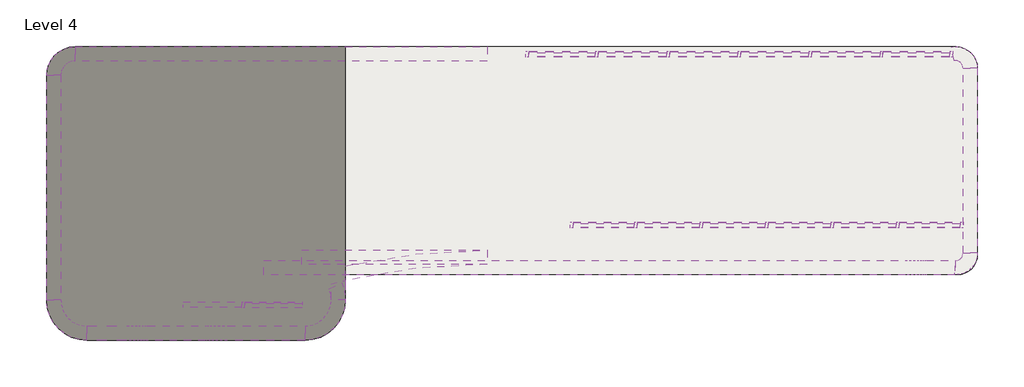
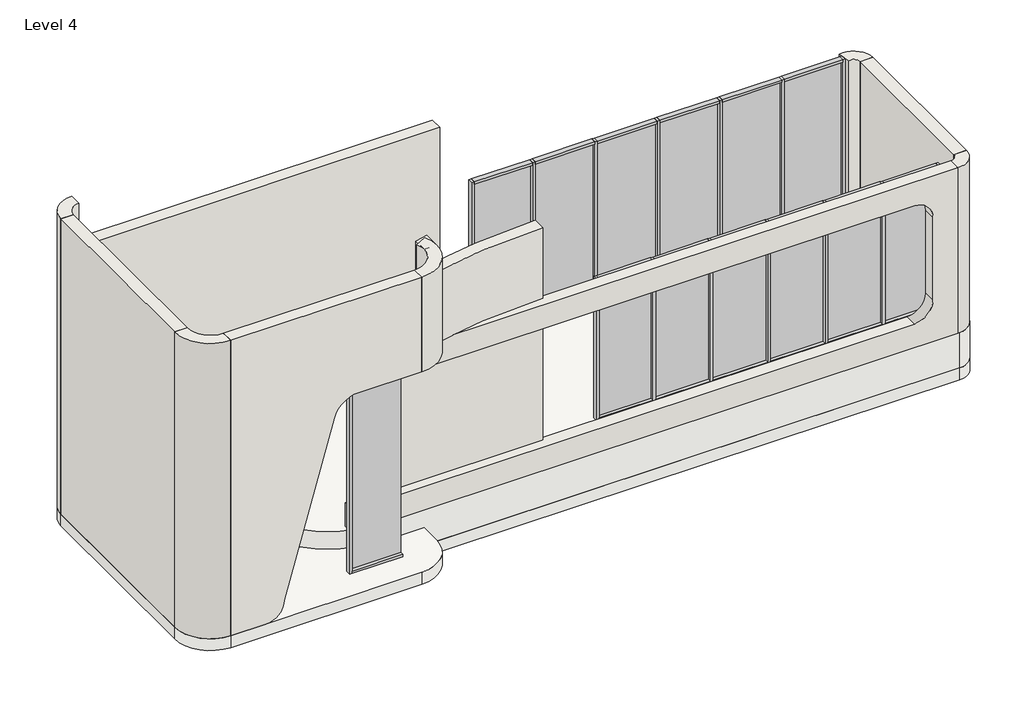
# One storey, incomplete: 41 members, 13 plates, 13 walls, 3 slabs.
"""IFC4 building model written with IfcOpenShell, lengths in millimetres."""

from ifc_helpers import new_model, si_unit, point, frame, frame_2d, origin, place, context, project, spatial, polyline, circle_curve, trimmed, segment, composite_curve, outline, extrude, faceted_brep, transform, mapped, element, save
from ifc_brep_helpers import plane_surface, cylinder_surface, revolved_surface, advanced_brep
from components import member_810865a4, member_4d31274b, member_efb4c79c, member_f6f550b4, member_9ad43860, member_f11946c0, member_9e61c091, member_45b72dba, member_ecd02cc6, member_9771a04b, member_bcb6a316, system_panel_glazed_7496e499, system_panel_glazed_f24f7e4d, system_panel_glazed_963389ce, system_panel_glazed_dc9dfaf4, system_panel_glazed_d8816065

model = new_model("IFC4")

# Units and contexts
model_context = context("Model", 3, world=origin())
ifc_project = project(units=[si_unit("LENGTHUNIT", "METRE", prefix="MILLI")], contexts=[model_context])

# Site, building, storey
site = spatial("IfcSite", under=ifc_project)
building = spatial("IfcBuilding", under=site)
storey = spatial("IfcBuildingStorey", under=building, Name="Level 4", Elevation=9144.0)

# Members
placement = place(None, origin())
member_shape = member_810865a4(model_context)
element("IfcMember", 1, ObjectType="Rectangular Mullion : 2.5\" x 5\" rectangular", at=placement, inside=storey, context=model_context, shape_type="MappedRepresentation", body=[
    mapped(member_shape, transform((-2482.72102, 10552.4053975, 10820.4), x_axis=(1.0, 0.0, 0.0), y_axis=(0.0, -1.0, 0.0), z_axis=(0.0, 0.0, -1.0))),
])
element("IfcMember", 2, ObjectType="Rectangular Mullion : 2.5\" x 5\" rectangular", at=placement, inside=storey, context=model_context, shape_type="MappedRepresentation", body=[
    mapped(member_shape, transform((-1082.1055914, 10552.4053975, 10820.4), x_axis=(1.0, 0.0, 0.0), y_axis=(0.0, -1.0, 0.0), z_axis=(0.0, 0.0, -1.0))),
])
element("IfcMember", 3, ObjectType="Rectangular Mullion : 2.5\" x 5\" rectangular", at=placement, inside=storey, context=model_context, shape_type="MappedRepresentation", body=[
    mapped(member_shape, transform((318.5098372, 10552.4053975, 10820.4), x_axis=(1.0, 0.0, 0.0), y_axis=(0.0, -1.0, 0.0), z_axis=(0.0, 0.0, -1.0))),
])
element("IfcMember", 4, ObjectType="Rectangular Mullion : 2.5\" x 5\" rectangular", at=placement, inside=storey, context=model_context, shape_type="MappedRepresentation", body=[
    mapped(member_shape, transform((1719.1252657, 10552.4053975, 10820.4), x_axis=(1.0, 0.0, 0.0), y_axis=(0.0, -1.0, 0.0), z_axis=(0.0, 0.0, -1.0))),
])
element("IfcMember", 5, ObjectType="Rectangular Mullion : 2.5\" x 5\" rectangular", at=placement, inside=storey, context=model_context, shape_type="MappedRepresentation", body=[
    mapped(member_shape, transform((3119.7406943, 10552.4053975, 10820.4), x_axis=(1.0, 0.0, 0.0), y_axis=(0.0, -1.0, 0.0), z_axis=(0.0, 0.0, -1.0))),
])
member_2_shape = member_4d31274b(model_context)
element("IfcMember", 6, ObjectType="Rectangular Mullion : 2.5\" x 5\" rectangular", at=placement, inside=storey, context=model_context, shape_type="MappedRepresentation", body=[
    mapped(member_2_shape, transform((4520.3561229, 10552.4053975, 10820.4), x_axis=(1.0, 0.0, 0.0), y_axis=(0.0, -1.0, 0.0), z_axis=(0.0, 0.0, -1.0))),
])
element("IfcMember", 7, ObjectType="Rectangular Mullion : 2.5\" x 5\" rectangular", at=placement, inside=storey, context=model_context, shape_type="MappedRepresentation", body=[
    mapped(member_2_shape, transform((-3883.3364486, 10552.4053975, 14478.0), x_axis=(-1.0, 0.0, 0.0), y_axis=(0.0, -1.0, 0.0), z_axis=(0.0, 0.0, 1.0))),
])
member_3_shape = member_efb4c79c(model_context)
element("IfcMember", 8, ObjectType="Rectangular Mullion : 2.5\" x 5\" rectangular", at=placement, inside=storey, context=model_context, shape_type="MappedRepresentation", body=[
    mapped(member_3_shape, transform((4456.8561229, 10552.4053975, 14478.0), x_axis=(0.0, 0.0, 1.0), y_axis=(0.0, -1.0, 0.0), z_axis=(1.0, 0.0, 0.0))),
])
element("IfcMember", 9, ObjectType="Rectangular Mullion : 2.5\" x 5\" rectangular", at=placement, inside=storey, context=model_context, shape_type="MappedRepresentation", body=[
    mapped(member_3_shape, transform((-2514.47102, 10552.4053975, 14478.0), x_axis=(0.0, 0.0, 1.0), y_axis=(0.0, -1.0, 0.0), z_axis=(1.0, 0.0, 0.0))),
])
member_4_shape = member_f6f550b4(model_context)
element("IfcMember", 10, ObjectType="Rectangular Mullion : 2.5\" x 5\" rectangular", at=placement, inside=storey, context=model_context, shape_type="MappedRepresentation", body=[
    mapped(member_4_shape, transform((-1113.8555914, 10552.4053975, 14478.0), x_axis=(0.0, 0.0, 1.0), y_axis=(0.0, -1.0, 0.0), z_axis=(1.0, 0.0, 0.0))),
])
element("IfcMember", 11, ObjectType="Rectangular Mullion : 2.5\" x 5\" rectangular", at=placement, inside=storey, context=model_context, shape_type="MappedRepresentation", body=[
    mapped(member_4_shape, transform((286.7598372, 10552.4053975, 14478.0), x_axis=(0.0, 0.0, 1.0), y_axis=(0.0, -1.0, 0.0), z_axis=(1.0, 0.0, 0.0))),
])
element("IfcMember", 12, ObjectType="Rectangular Mullion : 2.5\" x 5\" rectangular", at=placement, inside=storey, context=model_context, shape_type="MappedRepresentation", body=[
    mapped(member_4_shape, transform((1687.3752657, 10552.4053975, 14478.0), x_axis=(0.0, 0.0, 1.0), y_axis=(0.0, -1.0, 0.0), z_axis=(1.0, 0.0, 0.0))),
])
element("IfcMember", 13, ObjectType="Rectangular Mullion : 2.5\" x 5\" rectangular", at=placement, inside=storey, context=model_context, shape_type="MappedRepresentation", body=[
    mapped(member_4_shape, transform((3087.9906943, 10552.4053975, 14478.0), x_axis=(0.0, 0.0, 1.0), y_axis=(0.0, -1.0, 0.0), z_axis=(1.0, 0.0, 0.0))),
])
element("IfcMember", 14, ObjectType="Rectangular Mullion : 2.5\" x 5\" rectangular", at=placement, inside=storey, context=model_context, shape_type="MappedRepresentation", body=[
    mapped(member_3_shape, transform((-3819.8364486, 10552.4053975, 10820.4), x_axis=(0.0, 0.0, -1.0), y_axis=(0.0, -1.0, 0.0), z_axis=(-1.0, 0.0, 0.0))),
])
element("IfcMember", 15, ObjectType="Rectangular Mullion : 2.5\" x 5\" rectangular", at=placement, inside=storey, context=model_context, shape_type="MappedRepresentation", body=[
    mapped(member_3_shape, transform((3151.4906943, 10552.4053975, 10820.4), x_axis=(0.0, 0.0, -1.0), y_axis=(0.0, -1.0, 0.0), z_axis=(-1.0, 0.0, 0.0))),
])
element("IfcMember", 16, ObjectType="Rectangular Mullion : 2.5\" x 5\" rectangular", at=placement, inside=storey, context=model_context, shape_type="MappedRepresentation", body=[
    mapped(member_4_shape, transform((-2450.97102, 10552.4053975, 10820.4), x_axis=(0.0, 0.0, -1.0), y_axis=(0.0, -1.0, 0.0), z_axis=(-1.0, 0.0, 0.0))),
])
element("IfcMember", 17, ObjectType="Rectangular Mullion : 2.5\" x 5\" rectangular", at=placement, inside=storey, context=model_context, shape_type="MappedRepresentation", body=[
    mapped(member_4_shape, transform((-1050.3555914, 10552.4053975, 10820.4), x_axis=(0.0, 0.0, -1.0), y_axis=(0.0, -1.0, 0.0), z_axis=(-1.0, 0.0, 0.0))),
])
element("IfcMember", 18, ObjectType="Rectangular Mullion : 2.5\" x 5\" rectangular", at=placement, inside=storey, context=model_context, shape_type="MappedRepresentation", body=[
    mapped(member_4_shape, transform((350.2598372, 10552.4053975, 10820.4), x_axis=(0.0, 0.0, -1.0), y_axis=(0.0, -1.0, 0.0), z_axis=(-1.0, 0.0, 0.0))),
])
element("IfcMember", 19, ObjectType="Rectangular Mullion : 2.5\" x 5\" rectangular", at=placement, inside=storey, context=model_context, shape_type="MappedRepresentation", body=[
    mapped(member_4_shape, transform((1750.8752657, 10552.4053975, 10820.4), x_axis=(0.0, 0.0, -1.0), y_axis=(0.0, -1.0, 0.0), z_axis=(-1.0, 0.0, 0.0))),
])
member_5_shape = member_9ad43860(model_context)
element("IfcMember", 20, ObjectType="Rectangular Mullion : 2.5\" x 5\" rectangular", at=placement, inside=storey, context=model_context, shape_type="MappedRepresentation", body=[
    mapped(member_5_shape, transform((4234.1857714, 14210.0053975, 15087.6), x_axis=(0.0, 0.0, 1.0), y_axis=(0.0, -1.0, 0.0), z_axis=(1.0, 0.0, 0.0))),
])
element("IfcMember", 21, ObjectType="Rectangular Mullion : 2.5\" x 5\" rectangular", at=placement, inside=storey, context=model_context, shape_type="MappedRepresentation", body=[
    mapped(member_5_shape, transform((-3342.6529449, 14210.0053975, 15087.6), x_axis=(0.0, 0.0, 1.0), y_axis=(0.0, -1.0, 0.0), z_axis=(1.0, 0.0, 0.0))),
])
member_6_shape = member_f11946c0(model_context)
element("IfcMember", 22, ObjectType="Rectangular Mullion : 2.5\" x 5\" rectangular", at=placement, inside=storey, context=model_context, shape_type="MappedRepresentation", body=[
    mapped(member_6_shape, transform((-1820.9352016, 14210.0053975, 15087.6), x_axis=(0.0, 0.0, 1.0), y_axis=(0.0, -1.0, 0.0), z_axis=(1.0, 0.0, 0.0))),
])
element("IfcMember", 23, ObjectType="Rectangular Mullion : 2.5\" x 5\" rectangular", at=placement, inside=storey, context=model_context, shape_type="MappedRepresentation", body=[
    mapped(member_6_shape, transform((-299.2174584, 14210.0053975, 15087.6), x_axis=(0.0, 0.0, 1.0), y_axis=(0.0, -1.0, 0.0), z_axis=(1.0, 0.0, 0.0))),
])
element("IfcMember", 24, ObjectType="Rectangular Mullion : 2.5\" x 5\" rectangular", at=placement, inside=storey, context=model_context, shape_type="MappedRepresentation", body=[
    mapped(member_6_shape, transform((1222.5002849, 14210.0053975, 15087.6), x_axis=(0.0, 0.0, 1.0), y_axis=(0.0, -1.0, 0.0), z_axis=(1.0, 0.0, 0.0))),
])
element("IfcMember", 25, ObjectType="Rectangular Mullion : 2.5\" x 5\" rectangular", at=placement, inside=storey, context=model_context, shape_type="MappedRepresentation", body=[
    mapped(member_6_shape, transform((2744.2180281, 14210.0053975, 15087.6), x_axis=(0.0, 0.0, 1.0), y_axis=(0.0, -1.0, 0.0), z_axis=(1.0, 0.0, 0.0))),
])
element("IfcMember", 26, ObjectType="Rectangular Mullion : 2.5\" x 5\" rectangular", at=placement, inside=storey, context=model_context, shape_type="MappedRepresentation", body=[
    mapped(member_5_shape, transform((-4769.1206882, 14210.0053975, 10820.4), x_axis=(0.0, 0.0, -1.0), y_axis=(0.0, -1.0, 0.0), z_axis=(-1.0, 0.0, 0.0))),
])
element("IfcMember", 27, ObjectType="Rectangular Mullion : 2.5\" x 5\" rectangular", at=placement, inside=storey, context=model_context, shape_type="MappedRepresentation", body=[
    mapped(member_5_shape, transform((2807.7180281, 14210.0053975, 10820.4), x_axis=(0.0, 0.0, -1.0), y_axis=(0.0, -1.0, 0.0), z_axis=(-1.0, 0.0, 0.0))),
])
element("IfcMember", 28, ObjectType="Rectangular Mullion : 2.5\" x 5\" rectangular", at=placement, inside=storey, context=model_context, shape_type="MappedRepresentation", body=[
    mapped(member_6_shape, transform((-3279.1529449, 14210.0053975, 10820.4), x_axis=(0.0, 0.0, -1.0), y_axis=(0.0, -1.0, 0.0), z_axis=(-1.0, 0.0, 0.0))),
])
element("IfcMember", 29, ObjectType="Rectangular Mullion : 2.5\" x 5\" rectangular", at=placement, inside=storey, context=model_context, shape_type="MappedRepresentation", body=[
    mapped(member_6_shape, transform((-1757.4352016, 14210.0053975, 10820.4), x_axis=(0.0, 0.0, -1.0), y_axis=(0.0, -1.0, 0.0), z_axis=(-1.0, 0.0, 0.0))),
])
element("IfcMember", 30, ObjectType="Rectangular Mullion : 2.5\" x 5\" rectangular", at=placement, inside=storey, context=model_context, shape_type="MappedRepresentation", body=[
    mapped(member_6_shape, transform((-235.7174584, 14210.0053975, 10820.4), x_axis=(0.0, 0.0, -1.0), y_axis=(0.0, -1.0, 0.0), z_axis=(-1.0, 0.0, 0.0))),
])
element("IfcMember", 31, ObjectType="Rectangular Mullion : 2.5\" x 5\" rectangular", at=placement, inside=storey, context=model_context, shape_type="MappedRepresentation", body=[
    mapped(member_6_shape, transform((1286.0002849, 14210.0053975, 10820.4), x_axis=(0.0, 0.0, -1.0), y_axis=(0.0, -1.0, 0.0), z_axis=(-1.0, 0.0, 0.0))),
])
member_7_shape = member_9e61c091(model_context)
element("IfcMember", 32, ObjectType="Rectangular Mullion : 2.5\" x 5\" rectangular", at=placement, inside=storey, context=model_context, shape_type="MappedRepresentation", body=[
    mapped(member_7_shape, transform((-3310.9029449, 14210.0053975, 10820.4), x_axis=(1.0, 0.0, 0.0), y_axis=(0.0, -1.0, 0.0), z_axis=(0.0, 0.0, -1.0))),
])
element("IfcMember", 33, ObjectType="Rectangular Mullion : 2.5\" x 5\" rectangular", at=placement, inside=storey, context=model_context, shape_type="MappedRepresentation", body=[
    mapped(member_7_shape, transform((-1789.1852016, 14210.0053975, 10820.4), x_axis=(1.0, 0.0, 0.0), y_axis=(0.0, -1.0, 0.0), z_axis=(0.0, 0.0, -1.0))),
])
element("IfcMember", 34, ObjectType="Rectangular Mullion : 2.5\" x 5\" rectangular", at=placement, inside=storey, context=model_context, shape_type="MappedRepresentation", body=[
    mapped(member_7_shape, transform((-267.4674584, 14210.0053975, 10820.4), x_axis=(1.0, 0.0, 0.0), y_axis=(0.0, -1.0, 0.0), z_axis=(0.0, 0.0, -1.0))),
])
element("IfcMember", 35, ObjectType="Rectangular Mullion : 2.5\" x 5\" rectangular", at=placement, inside=storey, context=model_context, shape_type="MappedRepresentation", body=[
    mapped(member_7_shape, transform((1254.2502849, 14210.0053975, 10820.4), x_axis=(1.0, 0.0, 0.0), y_axis=(0.0, -1.0, 0.0), z_axis=(0.0, 0.0, -1.0))),
])
element("IfcMember", 36, ObjectType="Rectangular Mullion : 2.5\" x 5\" rectangular", at=placement, inside=storey, context=model_context, shape_type="MappedRepresentation", body=[
    mapped(member_7_shape, transform((2775.9680281, 14210.0053975, 10820.4), x_axis=(1.0, 0.0, 0.0), y_axis=(0.0, -1.0, 0.0), z_axis=(0.0, 0.0, -1.0))),
])
member_8_shape = member_45b72dba(model_context)
element("IfcMember", 37, ObjectType="Rectangular Mullion : 2.5\" x 5\" rectangular", at=placement, inside=storey, context=model_context, shape_type="MappedRepresentation", body=[
    mapped(member_8_shape, transform((4297.6857714, 14210.0053975, 10820.4), x_axis=(1.0, 0.0, 0.0), y_axis=(0.0, -1.0, 0.0), z_axis=(0.0, 0.0, -1.0))),
])
element("IfcMember", 38, ObjectType="Rectangular Mullion : 2.5\" x 5\" rectangular", at=placement, inside=storey, context=model_context, shape_type="MappedRepresentation", body=[
    mapped(member_8_shape, transform((-4832.6206882, 14210.0053975, 15087.6), x_axis=(-1.0, 0.0, 0.0), y_axis=(0.0, -1.0, 0.0), z_axis=(0.0, 0.0, 1.0))),
])
member_9_shape = member_ecd02cc6(model_context)
element("IfcMember", 39, ObjectType="Rectangular Mullion : 2.5\" x 5\" rectangular", at=placement, inside=storey, context=model_context, shape_type="MappedRepresentation", body=[
    mapped(member_9_shape, transform((-10872.9017879, 8841.0808402, 10363.2), x_axis=(1.0, 0.0, 0.0), y_axis=(0.0, -1.0, 0.0), z_axis=(0.0, 0.0, -1.0))),
])
member_10_shape = member_9771a04b(model_context)
element("IfcMember", 40, ObjectType="Rectangular Mullion : 2.5\" x 5\" rectangular", at=placement, inside=storey, context=model_context, shape_type="MappedRepresentation", body=[
    mapped(member_10_shape, transform((-10841.1517879, 8841.0808402, 10363.2), x_axis=(0.0, 0.0, -1.0), y_axis=(0.0, -1.0, 0.0), z_axis=(-1.0, 0.0, 0.0))),
])
member_11_shape = member_bcb6a316(model_context)
element("IfcMember", 41, ObjectType="Rectangular Mullion : 2.5\" x 5\" rectangular", at=placement, inside=storey, context=model_context, shape_type="MappedRepresentation", body=[
    mapped(member_11_shape, transform((-10904.6517879, 8841.0808402, 16374.9116741), x_axis=(0.0, 0.0, 1.0), y_axis=(0.0, -1.0, 0.0), z_axis=(1.0, 0.0, 0.0))),
])

# Plates
system_panel_glazed_shape = system_panel_glazed_7496e499(model_context)
element("IfcPlate", 42, ObjectType="System Panel : Glazed", at=placement, inside=storey, context=model_context, shape_type="MappedRepresentation", body=[
    mapped(system_panel_glazed_shape, transform((-3167.1537343, 10552.4053975, 10883.9), x_axis=(1.0, 0.0, 0.0), y_axis=(0.0, 1.0, 0.0), z_axis=(0.0, 0.0, 1.0))),
])
element("IfcPlate", 43, ObjectType="System Panel : Glazed", at=placement, inside=storey, context=model_context, shape_type="MappedRepresentation", body=[
    mapped(system_panel_glazed_shape, transform((3804.1734086, 10552.4053975, 10883.9), x_axis=(1.0, 0.0, 0.0), y_axis=(0.0, 1.0, 0.0), z_axis=(0.0, 0.0, 1.0))),
])
system_panel_glazed_2_shape = system_panel_glazed_f24f7e4d(model_context)
element("IfcPlate", 44, ObjectType="System Panel : Glazed", at=placement, inside=storey, context=model_context, shape_type="MappedRepresentation", body=[
    mapped(system_panel_glazed_2_shape, transform((-1782.4133057, 10552.4053975, 10883.9), x_axis=(1.0, 0.0, 0.0), y_axis=(0.0, 1.0, 0.0), z_axis=(0.0, 0.0, 1.0))),
])
element("IfcPlate", 45, ObjectType="System Panel : Glazed", at=placement, inside=storey, context=model_context, shape_type="MappedRepresentation", body=[
    mapped(system_panel_glazed_2_shape, transform((-381.7978771, 10552.4053975, 10883.9), x_axis=(1.0, 0.0, 0.0), y_axis=(0.0, 1.0, 0.0), z_axis=(0.0, 0.0, 1.0))),
])
element("IfcPlate", 46, ObjectType="System Panel : Glazed", at=placement, inside=storey, context=model_context, shape_type="MappedRepresentation", body=[
    mapped(system_panel_glazed_2_shape, transform((1018.8175515, 10552.4053975, 10883.9), x_axis=(1.0, 0.0, 0.0), y_axis=(0.0, 1.0, 0.0), z_axis=(0.0, 0.0, 1.0))),
])
element("IfcPlate", 47, ObjectType="System Panel : Glazed", at=placement, inside=storey, context=model_context, shape_type="MappedRepresentation", body=[
    mapped(system_panel_glazed_2_shape, transform((2419.43298, 10552.4053975, 10883.9), x_axis=(1.0, 0.0, 0.0), y_axis=(0.0, 1.0, 0.0), z_axis=(0.0, 0.0, 1.0))),
])
system_panel_glazed_3_shape = system_panel_glazed_963389ce(model_context)
element("IfcPlate", 48, ObjectType="System Panel : Glazed", at=placement, inside=storey, context=model_context, shape_type="MappedRepresentation", body=[
    mapped(system_panel_glazed_3_shape, transform((-4055.8868165, 14210.0053975, 10883.9), x_axis=(1.0, 0.0, 0.0), y_axis=(0.0, 1.0, 0.0), z_axis=(0.0, 0.0, 1.0))),
])
element("IfcPlate", 49, ObjectType="System Panel : Glazed", at=placement, inside=storey, context=model_context, shape_type="MappedRepresentation", body=[
    mapped(system_panel_glazed_3_shape, transform((3520.9518998, 14210.0053975, 10883.9), x_axis=(1.0, 0.0, 0.0), y_axis=(0.0, 1.0, 0.0), z_axis=(0.0, 0.0, 1.0))),
])
system_panel_glazed_4_shape = system_panel_glazed_dc9dfaf4(model_context)
element("IfcPlate", 50, ObjectType="System Panel : Glazed", at=placement, inside=storey, context=model_context, shape_type="MappedRepresentation", body=[
    mapped(system_panel_glazed_4_shape, transform((-2550.0440733, 14210.0053975, 10883.9), x_axis=(1.0, 0.0, 0.0), y_axis=(0.0, 1.0, 0.0), z_axis=(0.0, 0.0, 1.0))),
])
element("IfcPlate", 51, ObjectType="System Panel : Glazed", at=placement, inside=storey, context=model_context, shape_type="MappedRepresentation", body=[
    mapped(system_panel_glazed_4_shape, transform((-1028.32633, 14210.0053975, 10883.9), x_axis=(1.0, 0.0, 0.0), y_axis=(0.0, 1.0, 0.0), z_axis=(0.0, 0.0, 1.0))),
])
element("IfcPlate", 52, ObjectType="System Panel : Glazed", at=placement, inside=storey, context=model_context, shape_type="MappedRepresentation", body=[
    mapped(system_panel_glazed_4_shape, transform((493.3914133, 14210.0053975, 10883.9), x_axis=(1.0, 0.0, 0.0), y_axis=(0.0, 1.0, 0.0), z_axis=(0.0, 0.0, 1.0))),
])
element("IfcPlate", 53, ObjectType="System Panel : Glazed", at=placement, inside=storey, context=model_context, shape_type="MappedRepresentation", body=[
    mapped(system_panel_glazed_4_shape, transform((2015.1091565, 14210.0053975, 10883.9), x_axis=(1.0, 0.0, 0.0), y_axis=(0.0, 1.0, 0.0), z_axis=(0.0, 0.0, 1.0))),
])
system_panel_glazed_5_shape = system_panel_glazed_d8816065(model_context)
element("IfcPlate", 54, ObjectType="System Panel : Glazed", at=placement, inside=storey, context=model_context, shape_type="MappedRepresentation", body=[
    mapped(system_panel_glazed_5_shape, transform((-10228.3767879, 8841.0808402, 10426.7), x_axis=(1.0, 0.0, 0.0), y_axis=(0.0, 1.0, 0.0), z_axis=(0.0, 0.0, 1.0))),
])

# Slabs
element("IfcSlab", 55, ObjectType="Generic - 12\"", at=placement, inside=storey, context=model_context, shape_type="SweptSolid", body=[
    extrude(outline(composite_curve([segment(trimmed(circle_curve(frame_2d((-9623.664807, 11924.0053975)), 2438.4), [point((-9623.664807, 9485.6053975))], [point((-9623.664807, 14362.4053975))], False, "CARTESIAN"), True, "CONTINUOUS"), segment(polyline([(-9623.664807, 14362.4053975), (4370.9874869, 14362.4053975)]), True, "CONTINUOUS"), segment(trimmed(circle_curve(frame_2d((4370.9874869, 13905.2053975)), 457.2), [point((4370.9874869, 14362.4053975))], [point((4828.1874869, 13905.2053975))], False, "CARTESIAN"), True, "CONTINUOUS"), segment(polyline([(4828.1874869, 13905.2053975), (4828.1874869, 9916.6576913)]), True, "CONTINUOUS"), segment(trimmed(circle_curve(frame_2d((4397.135193, 9916.6576913)), 431.0522938), [point((4828.1874869, 9916.6576913))], [point((4397.135193, 9485.6053975))], False, "CARTESIAN"), True, "CONTINUOUS"), segment(polyline([(4397.135193, 9485.6053975), (-9623.664807, 9485.6053975)]), True, "CONTINUOUS")], self_intersect=False)), frame((0.0, 0.0, 9601.2), z_axis=(0.0, 0.0, 1.0), x_axis=(1.0, 0.0, 0.0)), (0.0, 0.0, 1.0), 304.8),
])
element("IfcSlab", 56, ObjectType="Generic - 12\"", at=placement, inside=storey, context=model_context, shape_type="SweptSolid", body=[
    extrude(outline(composite_curve([segment(polyline([(-9552.1017879, 8079.0808402), (-14219.3697324, 8079.0808402)]), True, "CONTINUOUS"), segment(trimmed(circle_curve(frame_2d((-14219.3697324, 8942.4209117)), 863.3400716), [point((-14219.3697324, 8079.0808402))], [point((-15082.709804, 8942.4209117))], False, "CARTESIAN"), True, "CONTINUOUS"), segment(polyline([(-15082.709804, 8942.4209117), (-15082.709804, 13752.8053975)]), True, "CONTINUOUS"), segment(trimmed(circle_curve(frame_2d((-14473.109804, 13752.8053975)), 609.6), [point((-15082.709804, 13752.8053975))], [point((-14473.109804, 14362.4053975))], False, "CARTESIAN"), True, "CONTINUOUS"), segment(polyline([(-14473.109804, 14362.4053975), (-8688.7617163, 14362.4053975), (-8688.7617163, 8942.4209117)]), True, "CONTINUOUS"), segment(trimmed(circle_curve(frame_2d((-9552.1017879, 8942.4209117)), 863.3400716), [point((-8688.7617163, 8942.4209117))], [point((-9552.1017879, 8079.0808402))], False, "CARTESIAN"), True, "CONTINUOUS")], self_intersect=False)), frame((0.0, 0.0, 10058.4), z_axis=(0.0, 0.0, 1.0), x_axis=(1.0, 0.0, 0.0)), (0.0, 0.0, 1.0), 304.8),
])
element("IfcSlab", 57, ObjectType="Generic - 3'", at=placement, inside=storey, context=model_context, shape_type="SweptSolid", body=[
    extrude(outline(composite_curve([segment(trimmed(circle_curve(frame_2d((-9623.664807, 11924.0053975)), 2438.4), [point((-9623.664807, 9485.6053975))], [point((-9623.664807, 14362.4053975))], False, "CARTESIAN"), True, "CONTINUOUS"), segment(polyline([(-9623.664807, 14362.4053975), (4370.9874869, 14362.4053975)]), True, "CONTINUOUS"), segment(trimmed(circle_curve(frame_2d((4370.9874869, 13905.2053975)), 457.2), [point((4370.9874869, 14362.4053975))], [point((4828.1874869, 13905.2053975))], False, "CARTESIAN"), True, "CONTINUOUS"), segment(polyline([(4828.1874869, 13905.2053975), (4828.1874869, 9916.6576913)]), True, "CONTINUOUS"), segment(trimmed(circle_curve(frame_2d((4397.135193, 9916.6576913)), 431.0522938), [point((4828.1874869, 9916.6576913))], [point((4397.135193, 9485.6053975))], False, "CARTESIAN"), True, "CONTINUOUS"), segment(polyline([(4397.135193, 9485.6053975), (-9623.664807, 9485.6053975)]), True, "CONTINUOUS")], self_intersect=False)), frame((0.0, 0.0, 9906.0), z_axis=(0.0, 0.0, 1.0), x_axis=(1.0, 0.0, 0.0)), (0.0, 0.0, 1.0), 914.4),
])

# Walls
element("IfcWall", 58, ObjectType="Generic - 12\" white", at=placement, inside=storey, context=model_context, shape_type="SweptSolid", body=[
    extrude(outline(polyline([(-5661.264807, 9704.4209117), (-9623.664807, 9704.4209117), (-9623.664807, 10009.2209117), (-5661.264807, 10009.2209117), (-5661.264807, 9704.4209117)])), frame((0.0, 0.0, 10820.4), z_axis=(0.0, 0.0, 1.0), x_axis=(1.0, 0.0, 0.0)), (0.0, 0.0, 1.0), 3657.6),
])
element("IfcWall", 59, ObjectType="Generic - 12\" white", at=placement, inside=storey, context=model_context, shape_type="AdvancedBrep", body=[
    advanced_brep(
    [(-10433.4614611, 9481.707593, 14478.0), (3282.5385389, 9481.707593, 14478.0), (3739.7385389, 9481.707593, 14020.8), (3739.7385389, 9481.707593, 11887.2), (3282.5385389, 9481.707593, 11430.0), (-10433.4614611, 9481.707593, 11430.0), (-10433.4614611, 9481.707593, 10820.4), (4346.6848749, 9481.707593, 10820.4), (4346.6848749, 9481.707593, 15087.6), (-10433.4614611, 9481.707593, 15087.6), (-10433.4614611, 9786.507593, 14478.0), (-10433.4614611, 9786.507593, 15087.6), (4352.7755462, 9786.507593, 15087.6), (4352.7755462, 9786.507593, 10820.4), (-10433.4614611, 9786.507593, 10820.4), (-10433.4614611, 9786.507593, 11430.0), (3282.5385389, 9786.507593, 11430.0), (3739.7385389, 9786.507593, 11887.2), (3739.7385389, 9786.507593, 14020.8), (3282.5385389, 9786.507593, 14478.0)],
    [
        (0, 1),
        (1, 2, circle_curve(frame((3282.5385389, 9481.707593, 14020.8), z_axis=(0.0, 1.0, 0.0), x_axis=(-1.0, 0.0, 0.0)), 457.2)),
        (2, 3),
        (3, 4, circle_curve(frame((3282.5385389, 9481.707593, 11887.2), z_axis=(0.0, 1.0, 0.0), x_axis=(-1.0, 0.0, 0.0)), 457.2)),
        (4, 5),
        (5, 6),
        (6, 7),
        (7, 8),
        (8, 9),
        (9, 0),
        (10, 11),
        (11, 12),
        (12, 13),
        (13, 14),
        (14, 15),
        (15, 16),
        (16, 17, circle_curve(frame((3282.5385389, 9786.507593, 11887.2), z_axis=(0.0, -1.0, 0.0), x_axis=(-1.0, 0.0, 0.0)), 457.2)),
        (17, 18),
        (18, 19, circle_curve(frame((3282.5385389, 9786.507593, 14020.8), z_axis=(0.0, -1.0, 0.0), x_axis=(-1.0, 0.0, 0.0)), 457.2)),
        (19, 10),
        (6, 14),
        (13, 7),
        (8, 12),
        (11, 9),
        (10, 0),
        (19, 1),
        (18, 2),
        (17, 3),
        (16, 4),
        (15, 5),
    ],
    [
        plane_surface(frame((3282.5385389, 9481.707593, 14478.0), z_axis=(0.0, -1.0, 0.0), x_axis=(1.0, 0.0, 0.0))),
        plane_surface(frame((3282.5385389, 9786.507593, 14478.0), z_axis=(0.0, 1.0, 0.0), x_axis=(-1.0, 0.0, 0.0))),
        plane_surface(frame((-10433.4614611, 9481.707593, 10820.4), z_axis=(0.0, 0.0, -1.0), x_axis=(0.0, 1.0, 0.0))),
        plane_surface(frame((4349.3385389, 9481.707593, 15087.6), z_axis=(0.0, 0.0, 1.0), x_axis=(0.0, 1.0, 0.0))),
        plane_surface(frame((-10433.4614611, 9481.707593, 15087.6), z_axis=(-1.0, 0.0, 0.0), x_axis=(0.0, 1.0, 0.0))),
        plane_surface(frame((-10433.4614611, 9481.707593, 14478.0), z_axis=(0.0, 0.0, -1.0), x_axis=(0.0, 1.0, 0.0))),
        revolved_surface(polyline([(2825.3385389, 9786.507593, 14020.8), (2825.3385389, 9481.707593, 14020.8)]), (3282.5385389, 9786.507593, 14020.8), (0.0, 1.0, 0.0)),
        plane_surface(frame((3739.7385389, 9481.707593, 14020.8), z_axis=(-1.0, 0.0, 0.0), x_axis=(0.0, 1.0, 0.0))),
        revolved_surface(polyline([(2825.3385389, 9786.507593, 11887.2), (2825.3385389, 9481.707593, 11887.2)]), (3282.5385389, 9786.507593, 11887.2), (0.0, 1.0, 0.0)),
        plane_surface(frame((3282.5385389, 9481.707593, 11430.0), z_axis=(0.0, 0.0, 1.0), x_axis=(0.0, 1.0, 0.0))),
        plane_surface(frame((-10433.4614611, 9481.707593, 11430.0), z_axis=(-1.0, 0.0, 0.0), x_axis=(0.0, 1.0, 0.0))),
        plane_surface(frame((4346.6848749, 9481.707593, 9144.0), z_axis=(0.9998004092690277, -0.019978529112143678, 0.0), x_axis=(0.019978529112143678, 0.9998004092690277, 0.0))),
    ],
    [
        (0, [[1, 2, 3, 4, 5, 6, 7, 8, 9, 10]]),
        (1, [[11, 12, 13, 14, 15, 16, 17, 18, 19, 20]]),
        (2, [[-7, 21, -14, 22]]),
        (3, [[-9, 23, -12, 24]]),
        (4, [[-10, -24, -11, 25]]),
        (5, [[-1, -25, -20, 26]]),
        (6, [[-2, -26, -19, 27]]),
        (7, [[-3, -27, -18, 28]]),
        (8, [[-4, -28, -17, 29]]),
        (9, [[-5, -29, -16, 30]]),
        (10, [[-6, -30, -15, -21]]),
        (11, [[-8, -22, -13, -23]]),
    ],
),
])
element("IfcWall", 60, ObjectType="Generic - 12\" white", at=placement, inside=storey, context=model_context, shape_type="SweptSolid", body=[
    extrude(outline(polyline([(4825.1561229, 13907.657593), (4825.1561229, 9945.257593), (4520.3561229, 9945.257593), (4520.3561229, 13907.657593), (4825.1561229, 13907.657593)])), frame((0.0, 0.0, 10820.4), z_axis=(0.0, 0.0, 1.0), x_axis=(1.0, 0.0, 0.0)), (0.0, 0.0, 1.0), 4267.2),
])
element("IfcWall", 61, ObjectType="Generic - 12\" white", at=placement, inside=storey, context=model_context, shape_type="SweptSolid", body=[
    extrude(outline(composite_curve([segment(polyline([(4520.3561229, 9945.257593), (4825.1561229, 9945.257593)]), True, "CONTINUOUS"), segment(trimmed(circle_curve(frame_2d((4361.3734614, 9945.257593)), 463.7826615), [point((4825.1561229, 9945.257593))], [point((4346.6848749, 9481.707593))], False, "CARTESIAN"), True, "CONTINUOUS"), segment(polyline([(4346.6848749, 9481.707593), (4352.7755462, 9786.507593)]), True, "CONTINUOUS"), segment(trimmed(circle_curve(frame_2d((4361.3734614, 9945.257593)), 158.9826615), [point((4352.7755462, 9786.507593))], [point((4520.3561229, 9945.257593))], True, "CARTESIAN"), True, "CONTINUOUS")], self_intersect=False)), frame((0.0, 0.0, 10820.4), z_axis=(0.0, 0.0, 1.0), x_axis=(1.0, 0.0, 0.0)), (0.0, 0.0, 1.0), 4267.2),
])
element("IfcWall", 62, ObjectType="Generic - 12\" white", at=placement, inside=storey, context=model_context, shape_type="SweptSolid", body=[
    extrude(outline(composite_curve([segment(polyline([(4825.1561229, 13907.657593), (4520.3561229, 13907.657593)]), True, "CONTINUOUS"), segment(trimmed(circle_curve(frame_2d((4363.3582159, 13907.657593)), 156.997907), [point((4520.3561229, 13907.657593))], [point((4330.0340204, 14061.0780636))], True, "CARTESIAN"), True, "CONTINUOUS"), segment(polyline([(4330.0340204, 14061.0780636), (4265.3375224, 14358.9327314)]), True, "CONTINUOUS"), segment(trimmed(circle_curve(frame_2d((4363.3582159, 13907.657593)), 461.797907), [point((4265.3375224, 14358.9327314))], [point((4825.1561229, 13907.657593))], False, "CARTESIAN"), True, "CONTINUOUS")], self_intersect=False)), frame((0.0, 0.0, 10820.4), z_axis=(0.0, 0.0, 1.0), x_axis=(1.0, 0.0, 0.0)), (0.0, 0.0, 1.0), 4267.2),
])
element("IfcWall", 63, ObjectType="Generic - 12\" white", at=placement, inside=storey, context=model_context, shape_type="SweptSolid", body=[
    extrude(outline(polyline([(-15082.709804, 8942.4209117), (-15082.709804, 13752.8053975), (-14777.909804, 13752.8053975), (-14777.909804, 8942.4209117), (-15082.709804, 8942.4209117)])), frame((0.0, 0.0, 10363.2), z_axis=(0.0, 0.0, 1.0), x_axis=(1.0, 0.0, 0.0)), (0.0, 0.0, 1.0), 7620.0),
])
element("IfcWall", 64, ObjectType="Generic - 12\" white", at=placement, inside=storey, context=model_context, shape_type="SweptSolid", body=[
    extrude(outline(composite_curve([segment(polyline([(15544.8, -9552.1017879), (17983.2, -9552.1017879), (17983.2, -14219.3697324), (10363.2, -14219.3697324), (10363.2, -13362.1017879)]), True, "CONTINUOUS"), segment(trimmed(circle_curve(frame_2d((10820.4, -13362.1017879)), 457.2), [point((10363.2, -13362.1017879))], [point((10820.4, -12904.9017879))], False, "CARTESIAN"), True, "CONTINUOUS"), segment(polyline([(10820.4, -12904.9017879), (15087.6, -11685.7017879)]), True, "CONTINUOUS"), segment(trimmed(circle_curve(frame_2d((14906.9662824, -11053.4837762)), 657.516657), [point((15087.6, -11685.7017879))], [point((15544.8, -11213.1593938))], True, "CARTESIAN"), True, "CONTINUOUS"), segment(polyline([(15544.8, -11213.1593938), (15544.8, -9552.1017879)]), True, "CONTINUOUS")], self_intersect=False)), frame((0.0, 8079.0808402, 0.0), z_axis=(0.0, 1.0, 0.0), x_axis=(0.0, 0.0, 1.0)), (0.0, 0.0, 1.0), 304.8),
])
element("IfcWall", 65, ObjectType="Generic - 12\" white", at=placement, inside=storey, context=model_context, shape_type="SweptSolid", body=[
    extrude(outline(composite_curve([segment(polyline([(-8688.7617163, 9360.9202505), (-8688.7617163, 8942.4209117), (-8993.5617163, 8942.4209117), (-8993.5617163, 9287.1189889)]), True, "CONTINUOUS"), segment(trimmed(circle_curve(frame_2d((-5661.2648069, -3808.9886493)), 13513.4095611), [point((-8993.5617163, 9287.1189889))], [point((-8688.7617163, 9360.9202505))], False, "CARTESIAN"), True, "CONTINUOUS")], self_intersect=False)), frame((0.0, 0.0, 15680.745847), z_axis=(0.0, 0.0, 1.0), x_axis=(1.0, 0.0, 0.0)), (0.0, 0.0, 1.0), 2302.454153),
])
element("IfcWall", 66, ObjectType="Generic - 12\" white", at=placement, inside=storey, context=model_context, shape_type="AdvancedBrep", body=[
    advanced_brep(
    [(-9552.1017879, 8079.0808402, 17983.2), (-8766.9201676, 9301.372026, 17983.2), (-9044.1265267, 9174.6452549, 17983.2), (-9552.1017879, 8383.8808402, 17983.2), (-9552.1017879, 8079.0808402, 15541.5627052), (-9552.1017879, 8383.8808402, 15541.5627052), (-9044.1265267, 9174.6452549, 15541.5627052), (-8766.9201676, 9301.372026, 15541.5627052), (-9552.1017879, 8079.0808402, 15544.8), (-9552.1017879, 8383.8808402, 15544.8)],
    [
        (0, 1, circle_curve(frame((-9552.1017879, 8942.4209117, 17983.2), z_axis=(0.0, 0.0, 1.0), x_axis=(1.0, 0.0, 0.0)), 863.3400716)),
        (1, 2),
        (2, 3, circle_curve(frame((-9552.1017879, 8942.4209117, 17983.2), z_axis=(0.0, 0.0, -1.0), x_axis=(1.0, 0.0, 0.0)), 558.5400716)),
        (3, 0),
        (4, 5),
        (5, 6, circle_curve(frame((-9552.1017879, 8942.4209117, 15541.5627052), z_axis=(0.0, 0.0, 1.0), x_axis=(1.0, 0.0, 0.0)), 558.5400716)),
        (6, 7),
        (7, 4, circle_curve(frame((-9552.1017879, 8942.4209117, 15541.5627052), z_axis=(0.0, 0.0, -1.0), x_axis=(1.0, 0.0, 0.0)), 863.3400716)),
        (0, 8),
        (8, 4),
        (7, 1),
        (6, 2),
        (5, 9),
        (9, 3),
    ],
    [
        plane_surface(frame((-8688.7617163, 8942.4209117, 17983.2), z_axis=(0.0, 0.0, 1.0), x_axis=(0.0, 1.0, 0.0))),
        plane_surface(frame((-8688.7617163, 8942.4209117, 15541.5627052), z_axis=(0.0, 0.0, -1.0), x_axis=(0.0, -1.0, 0.0))),
        cylinder_surface(frame((-9552.1017879, 8942.4209117, 15541.5627052), z_axis=(0.0, 0.0, 1.0), x_axis=(1.0, 0.0, 0.0)), 863.3400716),
        plane_surface(frame((-8766.9201676, 9301.372026, 17983.2), z_axis=(-0.41577024633640397, 0.9094696818813511, 0.0), x_axis=(0.0, 0.0, -1.0))),
        revolved_surface(polyline([(-8993.561716299999, 8942.4209117, 15541.5627052), (-8993.561716299999, 8942.4209117, 17983.2)]), (-9552.1017879, 8942.4209117, 15541.5627052), (0.0, 0.0, -1.0)),
        plane_surface(frame((-9552.1017879, 8383.8808402, 17983.2), z_axis=(-1.0, 0.0, 0.0), x_axis=(0.0, 0.0, -1.0))),
    ],
    [
        (0, [[1, 2, 3, 4]]),
        (1, [[5, 6, 7, 8]]),
        (2, [[-1, 9, 10, -8, 11]]),
        (3, [[-2, -11, -7, 12]]),
        (4, [[-3, -12, -6, 13, 14]]),
        (5, [[-4, -14, -13, -5, -10, -9]]),
    ],
),
])
element("IfcWall", 67, ObjectType="Generic - 12\" white", at=placement, inside=storey, context=model_context, shape_type="SweptSolid", body=[
    extrude(outline(composite_curve([segment(polyline([(-15082.709804, 8942.4209117), (-14777.909804, 8942.4209117)]), True, "CONTINUOUS"), segment(trimmed(circle_curve(frame_2d((-14219.3697324, 8942.4209117)), 558.5400716), [point((-14777.909804, 8942.4209117))], [point((-14219.3697324, 8383.8808402))], True, "CARTESIAN"), True, "CONTINUOUS"), segment(polyline([(-14219.3697324, 8383.8808402), (-14219.3697324, 8079.0808402)]), True, "CONTINUOUS"), segment(trimmed(circle_curve(frame_2d((-14219.3697324, 8942.4209117)), 863.3400716), [point((-14219.3697324, 8079.0808402))], [point((-15082.709804, 8942.4209117))], False, "CARTESIAN"), True, "CONTINUOUS")], self_intersect=False)), frame((0.0, 0.0, 10363.2), z_axis=(0.0, 0.0, 1.0), x_axis=(1.0, 0.0, 0.0)), (0.0, 0.0, 1.0), 7620.0),
])
element("IfcWall", 68, ObjectType="Generic - 12\" white", at=placement, inside=storey, context=model_context, shape_type="AdvancedBrep", body=[
    advanced_brep(
    [(-14473.109804, 14362.4053975, 17983.2), (-15082.709804, 13752.8053975, 17983.2), (-14777.909804, 13752.8053975, 17983.2), (-14473.109804, 14057.6053975, 17983.2), (-14473.109804, 14362.4053975, 10363.2), (-14473.109804, 14057.6053975, 10363.2), (-14777.909804, 13752.8053975, 10363.2), (-15082.709804, 13752.8053975, 10363.2), (-14473.109804, 14362.4053975, 16859.2175276), (-14473.109804, 14057.6053975, 16859.2175276)],
    [
        (0, 1, circle_curve(frame((-14473.109804, 13752.8053975, 17983.2), z_axis=(0.0, 0.0, 1.0), x_axis=(1.0, 0.0, 0.0)), 609.6)),
        (1, 2),
        (2, 3, circle_curve(frame((-14473.109804, 13752.8053975, 17983.2), z_axis=(0.0, 0.0, -1.0), x_axis=(1.0, 0.0, 0.0)), 304.8)),
        (3, 0),
        (4, 5),
        (5, 6, circle_curve(frame((-14473.109804, 13752.8053975, 10363.2), z_axis=(0.0, 0.0, 1.0), x_axis=(1.0, 0.0, 0.0)), 304.8)),
        (6, 7),
        (7, 4, circle_curve(frame((-14473.109804, 13752.8053975, 10363.2), z_axis=(0.0, 0.0, -1.0), x_axis=(1.0, 0.0, 0.0)), 609.6)),
        (0, 8),
        (8, 4),
        (7, 1),
        (6, 2),
        (5, 9),
        (9, 3),
    ],
    [
        plane_surface(frame((-13863.509804, 13752.8053975, 17983.2), z_axis=(0.0, 0.0, 1.0), x_axis=(0.0, 1.0, 0.0))),
        plane_surface(frame((-13863.509804, 13752.8053975, 10363.2), z_axis=(0.0, 0.0, -1.0), x_axis=(0.0, -1.0, 0.0))),
        cylinder_surface(frame((-14473.109804, 13752.8053975, 10363.2), z_axis=(0.0, 0.0, 1.0), x_axis=(1.0, 0.0, 0.0)), 609.6),
        plane_surface(frame((-15082.709804, 13752.8053975, 17983.2), z_axis=(0.0, -1.0, 0.0), x_axis=(0.0, 0.0, -1.0))),
        revolved_surface(polyline([(-14168.309804, 13752.8053975, 10363.2), (-14168.309804, 13752.8053975, 17983.2)]), (-14473.109804, 13752.8053975, 10363.2), (0.0, 0.0, -1.0)),
        plane_surface(frame((-14473.109804, 14057.6053975, 17983.2), z_axis=(1.0, 0.0, 0.0), x_axis=(0.0, 0.0, -1.0))),
    ],
    [
        (0, [[1, 2, 3, 4]]),
        (1, [[5, 6, 7, 8]]),
        (2, [[-1, 9, 10, -8, 11]]),
        (3, [[-2, -11, -7, 12]]),
        (4, [[-3, -12, -6, 13, 14]]),
        (5, [[-4, -14, -13, -5, -10, -9]]),
    ],
),
])
element("IfcWall", 69, ObjectType="Generic - 12\" white", at=placement, inside=storey, context=model_context, shape_type="Brep", body=[
    faceted_brep([(-14473.109804, 14057.6053975, 10363.2), (-5661.264807, 14057.6053975, 10363.2), (-5661.264807, 14057.6053975, 10820.4), (-5661.264807, 14057.6053975, 16859.2175276), (-14473.109804, 14057.6053975, 16859.2175276), (-14473.109804, 14362.4053975, 10363.2), (-14473.109804, 14362.4053975, 16859.2175276), (-5661.264807, 14362.4053975, 16859.2175276), (-5661.264807, 14362.4053975, 10820.4), (-5661.264807, 14362.4053975, 10363.2)], [[[0, 1, 2, 3, 4]], [[5, 6, 7, 8, 9]], [[1, 0, 5, 9]], [[4, 3, 7, 6]], [[0, 4, 6, 5]], [[1, 9, 8, 7, 3, 2]]]),
])
element("IfcWall", 70, ObjectType="Generic - 12\" white", at=placement, inside=storey, context=model_context, shape_type="SweptSolid", body=[
    extrude(outline(composite_curve([segment(polyline([(-8688.7617163, 9360.9202505), (-8688.7617163, 9673.4880496)]), True, "CONTINUOUS"), segment(trimmed(circle_curve(frame_2d((-5661.2648069, -3808.9886493)), 13818.2095611), [point((-8688.7617163, 9673.4880496))], [point((-5661.264807, 10009.2209117))], False, "CARTESIAN"), True, "CONTINUOUS"), segment(polyline([(-5661.264807, 10009.2209117), (-5661.264807, 9704.4209117)]), True, "CONTINUOUS"), segment(trimmed(circle_curve(frame_2d((-5661.2648069, -3808.9886493)), 13513.4095611), [point((-5661.264807, 9704.4209117))], [point((-8688.7617163, 9360.9202505))], True, "CARTESIAN"), True, "CONTINUOUS")], self_intersect=False)), frame((0.0, 0.0, 15087.6), z_axis=(0.0, 0.0, 1.0), x_axis=(1.0, 0.0, 0.0)), (0.0, 0.0, 1.0), 1828.8),
])

save(model, "model.ifc")

# Revit data of these elements
# Type "Rectangular Mullion : 2.5\" x 5\" rectangular"
#   built-in parameter 1007304 = 0.416667 (stored number, unit not read)
#   built-in parameter 1007301 = 0.104167 (stored number, unit not read)
#   built-in parameter 1007300 = 0.104167 (stored number, unit not read)
# Type "System Panel : Glazed"
#   Construction Type Id = "GSP4R"
#   Analytic Construction = "1/8 in Pilkington single glazing"
#   Visual Light Transmittance = 0.9
#   Solar Heat Gain Coefficient = 0.86
#   Heat Transfer Coefficient (U) = 1.18115 BTU/(h·ft²·°F)
# Type "Generic - 12\""
#   Assembly Code = "B1010"
#   Function = 0
#   Layers, outside or top first: 1' - 0" "Door - Frame" (function 1)
# Type "Generic - 3'"
#   Assembly Code = "B1010"
#   Function = 0
#   Layers, outside or top first: 3' - 0" "Door - Frame" (function 1)
# Type "Generic - 12\" white"
#   Assembly Code = "B2010"
#   Layers, outside or top first: 1' - 0" "Door - Frame" (function 1)
# Elements 1, 2, 3, 4, 5, 6, 7, 8, 9, 10, 11, 12, 13, 14, 15, 16, 17, 18, 19, 20, 21, 22, 23, 24, 25, 26, 27, 28, 29, 30, 31, 32, 33, 34, 35, 36, 37, 38, 39, 40, 41 (IfcMember, "Rectangular Mullion : 2.5\" x 5\" rectangular")
#   Phase Created = New Construction
#   Materials on its faces: "Iron, Ductile"
# Elements 42, 43, 44, 45, 46, 47, 48, 49, 50, 51, 52, 53, 54 (IfcPlate, "System Panel : Glazed")
#   Phase Created = New Construction
#   Materials on its faces: "Glass"
# Element 55 (IfcSlab, "Generic - 12\"")
#   Height Offset From Level = 2' - 6"
#   Phase Created = New Construction
#   Materials on its faces: "Door - Frame"
# Element 56 (IfcSlab, "Generic - 12\"")
#   Height Offset From Level = 4' - 0"
#   Phase Created = New Construction
#   Materials on its faces: "Door - Frame"
# Element 57 (IfcSlab, "Generic - 3'")
#   Height Offset From Level = 5' - 6"
#   Phase Created = New Construction
#   Materials on its faces: "Door - Frame"
# Element 58 (IfcWall, "Generic - 12\" white")
#   built-in parameter 1001111 = 5' - 6"
#   Top Offset = 0' - 0"
#   Base Offset = 5' - 6"
#   Unconnected Height = 12' - 0"
#   wall height = 12' - 0"
#   Phase Created = New Construction
#   Base Constraint = Level 4
#   Materials on its faces: "Door - Frame"
# Elements 59, 60 (IfcWall, "Generic - 12\" white")
#   built-in parameter 1001111 = 5' - 6"
#   Top Offset = 0' - 0"
#   Base Offset = 5' - 6"
#   Unconnected Height = 14' - 0"
#   wall height = 14' - 0"
#   Phase Created = New Construction
#   Base Constraint = Level 4
#   Materials on its faces: "Door - Frame"
# Elements 61, 62 (IfcWall, "Generic - 12\" white")
#   built-in parameter 1001111 = 5' - 6"
#   Top Offset = 0' - 0"
#   Base Offset = 5' - 6"
#   Unconnected Height = 14' - 0"
#   wall height = 14' - 0"
#   Phase Created = New Construction
#   Materials on its faces: "Door - Frame"
# Elements 63, 64 (IfcWall, "Generic - 12\" white")
#   built-in parameter 1001111 = 4' - 0"
#   Top Offset = 0' - 0"
#   Base Offset = 4' - 0"
#   Unconnected Height = 25' - 0"
#   wall height = 25' - 0"
#   Phase Created = New Construction
#   Base Constraint = Level 4
#   Materials on its faces: "Door - Frame"
# Element 65 (IfcWall, "Generic - 12\" white")
#   built-in parameter 1001111 = 20' - 11.92586"
#   Top Offset = 0' - 0"
#   Base Offset = 20' - 11.92586"
#   Unconnected Height = 8' - 0.07414"
#   wall height = 8' - 0.07414"
#   Phase Created = New Construction
#   Base Constraint = Level 4
#   Materials on its faces: "Door - Frame"
# Element 66 (IfcWall, "Generic - 12\" white")
#   built-in parameter 1001111 = 20' - 11.87255"
#   Top Offset = 0' - 0"
#   Base Offset = 20' - 11.87255"
#   Unconnected Height = 8' - 0.12745"
#   wall height = 8' - 0.12745"
#   Phase Created = New Construction
#   Materials on its faces: "Door - Frame"
# Elements 67, 68 (IfcWall, "Generic - 12\" white")
#   built-in parameter 1001111 = 4' - 0"
#   Top Offset = 0' - 0"
#   Base Offset = 4' - 0"
#   Unconnected Height = 25' - 0"
#   wall height = 25' - 0"
#   Phase Created = New Construction
#   Materials on its faces: "Door - Frame"
# Element 69 (IfcWall, "Generic - 12\" white")
#   built-in parameter 1001111 = 4' - 0"
#   Top Offset = 0' - 0"
#   Base Offset = 4' - 0"
#   Unconnected Height = 21' - 3.74872"
#   wall height = 21' - 3.74872"
#   Phase Created = New Construction
#   Base Constraint = Level 4
#   Materials on its faces: "Door - Frame"
# Element 70 (IfcWall, "Generic - 12\" white")
#   built-in parameter 1001111 = 19' - 6"
#   Top Offset = 0' - 0"
#   Base Offset = 19' - 6"
#   Unconnected Height = 6' - 0"
#   wall height = 6' - 0"
#   Phase Created = New Construction
#   Materials on its faces: "Door - Frame"
# Materials
#   "Door - Frame": colour RGB 118 70 51, transparency 0, Cost = 0
#   "Iron, Ductile": class "Metal", colour RGB 0 0 0, transparency 0, Description = "Ductile cast iron", Cost = 0
#   "Glass": class "Glass", colour RGB 0 128 192, transparency 0.75, Description = "Soda Lime Glass", Cost = 0
